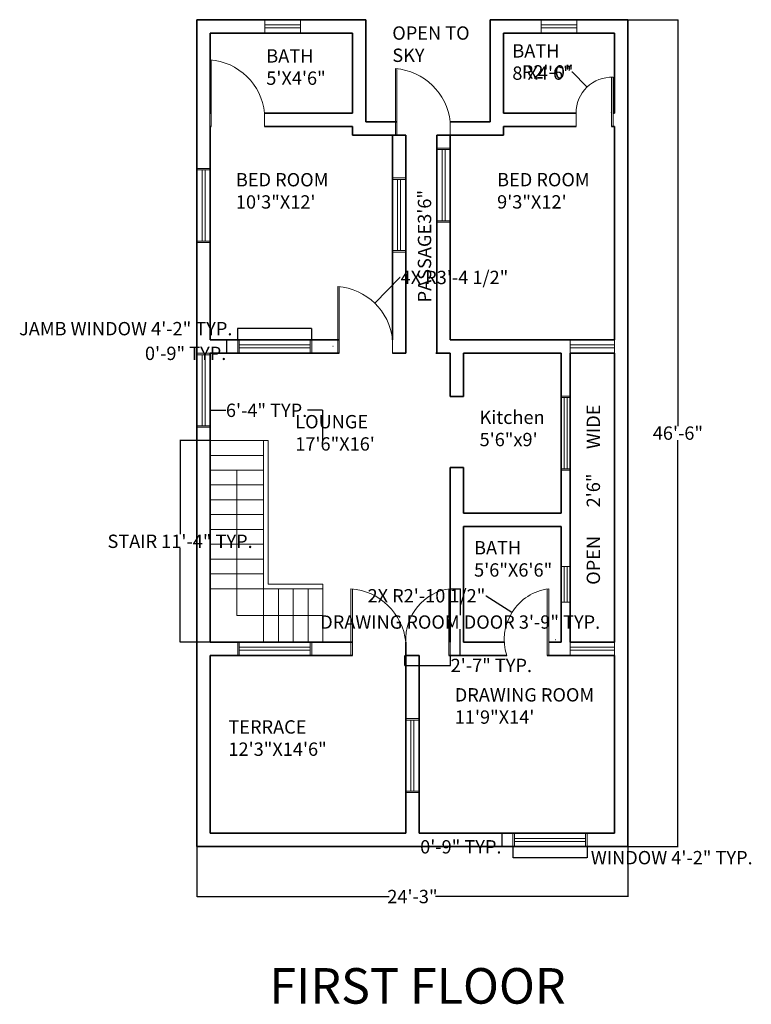
# Model space of a CAD drawing. Units: inches. Extents: x -56 to 1055, y -798 to 815.
# Tile 2 of 2: x 561 to 1055, y -756 to -91. Entities that reach past the tile are written whole.
import ezdxf

# ---------------------------------------------------------------- set-up
doc = ezdxf.new("R2010")
doc.units = ezdxf.units.IN
doc.header["$MEASUREMENT"] = 0
for name, color, linetype, lineweight in [('A-ANNO-DIMS', 2, 'Continuous', 18), ('A-ANNO-TEXT', 7, 'Continuous', 18), ('A-AREA-IDEN', 7, 'Continuous', 18), ('A-DOOR', 3, 'Continuous', 18), ('A-FLOR-STRS', 7, 'Continuous', 18), ('A-GLAZ', 4, 'Continuous', 18), ('A-WALL', 7, 'Continuous', 35)]:
    doc.layers.add(name, color=color, linetype=linetype, lineweight=lineweight)
doc.styles.get("Standard").update_dxf_attribs({"font": 'arial.ttf'})
doc.dimstyles.get("Standard").update_dxf_attribs({"dimtxt": 9, "dimasz": 0.18, "dimexe": 0.18, "dimexo": 0.0625, "dimgap": 0.09, "dimtad": 0, "dimtih": 1, "dimtoh": 1, "dimdec": 0, "dimzin": 0, "dimdsep": 46, "dimlunit": 3, "dimtxsty": 'Standard', "dimcen": 0.09, "dimadec": 0, "dimazin": 0, "dimtfac": 1, "dimtdec": 0, "dimtofl": 0, "dimtmove": 0, "dimatfit": 3, "dimfxl": 1, "dimtolj": 1, "dimtzin": 0, "dimarcsym": 0})

# ---------------------------------------------------------------- blocks, each defined once
blk = doc.blocks.new('door')
for p, q in [((432.11, -633.03), (432.11, -588.03)), ((433.11, -633.03), (433.11, -588.03)), ((469.11, -624.03), (469.11, -633.03))]:
    blk.add_line(p, q)
blk.add_arc((428.9, -628.35), 40.45, 6.12759, 85.44206)
blk = doc.blocks.new('WIN-50-FRAMED')
for p, q in [((0, 50), (9, 50)), ((0, 0), (0, 50)), ((0, 49), (9, 49)), ((3.5, 1), (3.5, 49)), ((5.5, 1), (5.5, 49)), ((9, 0), (9, 50)), ((0, 1), (9, 1)), ((0, 0), (9, 0))]:
    blk.add_line(p, q)
blk = doc.blocks.new('WIN-50-JAMB')
for p, q in [((0, 0), (0, 9)), ((1, 0), (1, 9)), ((49, 0), (49, 9)), ((50, 0), (50, 9)), ((1, 5.5), (49, 5.5)), ((1, 3.5), (49, 3.5))]:
    blk.add_line(p, q)
blk = doc.blocks.new('WIN-50-NARROW-WALL')
for p, q in [((0, 50), (6, 50)), ((0, 49), (6, 49)), ((2, 49), (2, 1)), ((4, 49), (4, 1)), ((0, 1), (6, 1)), ((0, 0), (6, 0))]:
    blk.add_line(p, q)
blk = doc.blocks.new('WIN-24-NARROW-WALL')
for p, q in [((0, 24), (6, 24)), ((2, 24), (2, 0)), ((4, 24), (4, 0)), ((0, 0), (6, 0))]:
    blk.add_line(p, q)
blk = doc.blocks.new('WIN-24-VENT')
for p, q in [((0, 0), (0, 9)), ((24, 0), (24, 9)), ((0, 5.5), (24, 5.5)), ((0, 3.5), (24, 3.5))]:
    blk.add_line(p, q)
blk = doc.blocks.new('DOOR-BATH-FRONT')
for p, q in [((29.04, 0), (29.04, 45)), ((30.04, 0), (30.04, 45)), ((0.04, 9), (0.04, 12.42))]:
    blk.add_line(p, q)
blk.add_arc((34.59, 10.71), 34.59, 97.55718, 198.03398)
blk = doc.blocks.new('DOOR-BATH-REAR')
for p, q in [((24, 0), (24, 33.14)), ((25, 0), (25, 33.14)), ((0, 0), (0, 9.51))]:
    blk.add_line(p, q)
blk.add_arc((23.91, 9.26), 23.91, 87.38829, 180.61249)
blk = doc.blocks.new('DOOR-DRAWING-ROOM')
for p, q in [((29.04, 0), (29.04, 45)), ((30.04, 0), (30.04, 45))]:
    blk.add_line(p, q)
blk.add_arc((34.59, 10.71), 34.59, 97.55718, 182.83167)
blk = doc.blocks.new('STAIR-RETURN')
for p, q in [((36, 136), (0, 136)), ((36, 136), (36, 36)), ((36, 136), (39, 136)), ((39, 136), (39, 39)), ((36, 126), (0, 126)), ((36, 116), (0, 116)), ((18, 116), (18, 18)), ((36, 106), (0, 106)), ((36, 96), (0, 96)), ((36, 86), (0, 86)), ((36, 76), (0, 76)), ((36, 66), (0, 66)), ((36, 56), (0, 56)), ((36, 46), (0, 46)), ((36, 36), (0, 36)), ((76, 36), (36, 36)), ((36, 36), (36, 0)), ((76, 39), (39, 39)), ((46, 36), (46, 0)), ((56, 36), (56, 0)), ((66, 36), (66, 0)), ((76, 36), (76, 39)), ((76, 36), (76, 0)), ((18, 18), (76, 18))]:
    blk.add_line(p, q)
blk = doc.blocks.new('WIN-30-OPENING')
for p, q in [((0, 0), (0, 9)), ((30, 9), (30, 0)), ((0, 5.5), (30, 5.5)), ((0, 3.5), (30, 3.5))]:
    blk.add_line(p, q)
blk = doc.blocks.new('WIN-30-SILL')
for p, q in [((0, 0), (0, 9)), ((30, 9), (30, 0)), ((0, 5.5), (30, 5.5)), ((0, 3.5), (30, 3.5)), ((0, 0), (30, 0))]:
    blk.add_line(p, q)
blk = doc.blocks.new('*D15')
at = {"layer": 'A-ANNO-DIMS', "color": 0, "lineweight": -2, "transparency": 16777216}
for p, q in [((893.64, -649.22), (893.64, -656.84)), ((943.64, -649.22), (943.64, -656.84)), ((893.82, -656.66), (943.46, -656.66)), ((943.64, -656.66), (943.82, -656.66))]:
    blk.add_line(p, q, dxfattribs=at)
at = {"layer": 'A-ANNO-DIMS', "color": 0, "transparency": 16777216}
for points in [[(893.82, -656.63), (893.82, -656.69), (893.64, -656.66)], [(943.46, -656.63), (943.46, -656.69), (943.64, -656.66)]]:
    blk.add_solid(points, dxfattribs=at)
at = {"layer": 'Defpoints', "color": 0, "transparency": 16777216}
for p in [(893.64, -649.16), (943.64, -649.16), (943.64, -656.66)]:
    blk.add_point(p, dxfattribs=at)
at = {"layer": 'A-ANNO-DIMS', "color": 0, "transparency": 16777216, "insert": (1000.85, -656.66), "char_height": 9, "attachment_point": 5}
blk.add_mtext('\\A1;WINDOW 4\'-2" TYP.', dxfattribs=at)
blk = doc.blocks.new('*D16')
at = {"layer": 'A-ANNO-DIMS', "color": 0, "lineweight": -2, "transparency": 16777216}
for p, q in [((893.58, -640.16), (885.96, -640.16)), ((886.14, -640.34), (886.14, -648.98)), ((893.58, -649.16), (885.96, -649.16)), ((886.14, -649.34), (885.96, -649.34)), ((886.14, -649.16), (886.14, -649.34))]:
    blk.add_line(p, q, dxfattribs=at)
at = {"layer": 'A-ANNO-DIMS', "color": 0, "transparency": 16777216}
for points in [[(886.11, -640.34), (886.17, -640.34), (886.14, -640.16)], [(886.11, -648.98), (886.17, -648.98), (886.14, -649.16)]]:
    blk.add_solid(points, dxfattribs=at)
at = {"layer": 'Defpoints', "color": 0, "transparency": 16777216}
for p in [(893.64, -640.16), (886.14, -649.16), (893.64, -649.16)]:
    blk.add_point(p, dxfattribs=at)
at = {"layer": 'A-ANNO-DIMS', "color": 0, "transparency": 16777216, "insert": (858.44, -649.34), "char_height": 9, "attachment_point": 5}
blk.add_mtext('\\A1;0\'-9" TYP.', dxfattribs=at)
blk = doc.blocks.new('*D19')
at = {"layer": 'A-ANNO-DIMS', "color": 0, "lineweight": -2, "transparency": 16777216}
for p, q in [((707.81, -299.66), (707.63, -299.66)), ((707.81, -307.1), (707.81, -299.48)), ((757.63, -299.66), (707.99, -299.66)), ((757.81, -307.1), (757.81, -299.48))]:
    blk.add_line(p, q, dxfattribs=at)
at = {"layer": 'A-ANNO-DIMS', "color": 0, "transparency": 16777216}
for points in [[(707.99, -299.63), (707.99, -299.69), (707.81, -299.66)], [(757.63, -299.63), (757.63, -299.69), (757.81, -299.66)]]:
    blk.add_solid(points, dxfattribs=at)
at = {"layer": 'Defpoints', "color": 0, "transparency": 16777216}
for p in [(707.81, -299.66), (707.81, -307.16), (757.81, -307.16)]:
    blk.add_point(p, dxfattribs=at)
at = {"layer": 'A-ANNO-DIMS', "color": 0, "transparency": 16777216, "insert": (632.18, -299.66), "char_height": 9, "attachment_point": 5}
blk.add_mtext('\\A1;JAMB WINDOW 4\'-2" TYP.', dxfattribs=at)
blk = doc.blocks.new('*D20')
at = {"layer": 'A-ANNO-DIMS', "color": 0, "lineweight": -2, "transparency": 16777216}
for p, q in [((707.75, -307.16), (700.13, -307.16)), ((700.31, -307.34), (700.31, -315.98)), ((707.75, -316.16), (700.13, -316.16)), ((700.31, -316.34), (700.13, -316.34)), ((700.31, -316.16), (700.31, -316.34))]:
    blk.add_line(p, q, dxfattribs=at)
at = {"layer": 'A-ANNO-DIMS', "color": 0, "transparency": 16777216}
for points in [[(700.28, -307.34), (700.34, -307.34), (700.31, -307.16)], [(700.28, -315.98), (700.34, -315.98), (700.31, -316.16)]]:
    blk.add_solid(points, dxfattribs=at)
at = {"layer": 'Defpoints', "color": 0, "transparency": 16777216}
for p in [(707.81, -307.16), (700.31, -316.16), (707.81, -316.16)]:
    blk.add_point(p, dxfattribs=at)
at = {"layer": 'A-ANNO-DIMS', "color": 0, "transparency": 16777216, "insert": (672.61, -316.34), "char_height": 9, "attachment_point": 5}
blk.add_mtext('\\A1;0\'-9" TYP.', dxfattribs=at)
blk = doc.blocks.new('*D31')
at = {"layer": 'A-ANNO-DIMS', "color": 0, "lineweight": -2, "transparency": 16777216}
for p, q in [((851.33, -475.16), (858.2, -475.16)), ((858.02, -475.34), (858.02, -492.91)), ((858.02, -519.98), (858.02, -502.41)), ((851.33, -520.16), (858.2, -520.16))]:
    blk.add_line(p, q, dxfattribs=at)
at = {"layer": 'A-ANNO-DIMS', "color": 0, "transparency": 16777216}
for points in [[(857.99, -475.34), (858.05, -475.34), (858.02, -475.16)], [(857.99, -519.98), (858.05, -519.98), (858.02, -520.16)]]:
    blk.add_solid(points, dxfattribs=at)
at = {"layer": 'Defpoints', "color": 0, "transparency": 16777216}
for p in [(851.27, -475.16), (858.02, -475.16), (851.27, -520.16)]:
    blk.add_point(p, dxfattribs=at)
at = {"layer": 'A-ANNO-DIMS', "color": 0, "transparency": 16777216, "insert": (858.02, -497.66), "char_height": 9, "attachment_point": 5}
blk.add_mtext('\\A1;DRAWING ROOM DOOR 3\'-9" TYP.', dxfattribs=at)
blk = doc.blocks.new('*D32')
at = {"layer": 'A-ANNO-DIMS', "color": 0, "lineweight": -2, "transparency": 16777216}
for p, q in [((820.38, -520.22), (820.38, -527.09)), ((851.27, -520.22), (851.27, -527.09)), ((820.56, -526.91), (851.09, -526.91)), ((851.27, -526.91), (851.45, -526.91))]:
    blk.add_line(p, q, dxfattribs=at)
at = {"layer": 'A-ANNO-DIMS', "color": 0, "transparency": 16777216}
for points in [[(820.56, -526.88), (820.56, -526.94), (820.38, -526.91)], [(851.09, -526.88), (851.09, -526.94), (851.27, -526.91)]]:
    blk.add_solid(points, dxfattribs=at)
at = {"layer": 'Defpoints', "color": 0, "transparency": 16777216}
for p in [(820.38, -520.16), (851.27, -520.16), (851.27, -526.91)]:
    blk.add_point(p, dxfattribs=at)
at = {"layer": 'A-ANNO-DIMS', "color": 0, "transparency": 16777216, "insert": (879.04, -526.91), "char_height": 9, "attachment_point": 5}
blk.add_mtext('\\A1;2\'-7" TYP.', dxfattribs=at)
blk = doc.blocks.new('*D33')
at = {"layer": 'A-ANNO-DIMS', "color": 0, "lineweight": -2, "transparency": 16777216}
for p, q in [((689.2, -375.16), (668.69, -375.16)), ((668.87, -375.34), (668.87, -438.42)), ((668.87, -510.98), (668.87, -447.9)), ((689.2, -511.16), (668.69, -511.16))]:
    blk.add_line(p, q, dxfattribs=at)
at = {"layer": 'A-ANNO-DIMS', "color": 0, "transparency": 16777216}
for points in [[(668.84, -375.34), (668.9, -375.34), (668.87, -375.16)], [(668.84, -510.98), (668.9, -510.98), (668.87, -511.16)]]:
    blk.add_solid(points, dxfattribs=at)
at = {"layer": 'Defpoints', "color": 0, "transparency": 16777216}
for p in [(668.87, -375.16), (689.27, -375.16), (689.27, -511.16)]:
    blk.add_point(p, dxfattribs=at)
at = {"layer": 'A-ANNO-DIMS', "color": 0, "transparency": 16777216, "insert": (668.87, -443.16), "char_height": 9, "attachment_point": 5}
blk.add_mtext('\\A1;STAIR 11\'-4" TYP.', dxfattribs=at)
blk = doc.blocks.new('*D34')
at = {"layer": 'A-ANNO-DIMS', "color": 0, "lineweight": -2, "transparency": 16777216}
for p, q in [((689.27, -375.1), (689.27, -354.58)), ((689.45, -354.76), (699.72, -354.76)), ((765.09, -354.76), (754.81, -354.76)), ((765.27, -375.1), (765.27, -354.58))]:
    blk.add_line(p, q, dxfattribs=at)
at = {"layer": 'A-ANNO-DIMS', "color": 0, "transparency": 16777216}
for points in [[(689.45, -354.73), (689.45, -354.79), (689.27, -354.76)], [(765.09, -354.73), (765.09, -354.79), (765.27, -354.76)]]:
    blk.add_solid(points, dxfattribs=at)
at = {"layer": 'Defpoints', "color": 0, "transparency": 16777216}
for p in [(765.27, -354.76), (689.27, -375.16), (765.27, -375.16)]:
    blk.add_point(p, dxfattribs=at)
at = {"layer": 'A-ANNO-DIMS', "color": 0, "transparency": 16777216, "insert": (727.27, -354.76), "char_height": 9, "attachment_point": 5}
blk.add_mtext('\\A1;6\'-4" TYP.', dxfattribs=at)
blk = doc.blocks.new('*D41')
at = {"layer": 'A-ANNO-DIMS', "color": 0, "lineweight": -2, "transparency": 16777216}
for p, q in [((680.27, -649.22), (680.27, -683.09)), ((971.27, -649.22), (971.27, -683.09)), ((680.45, -682.91), (810.14, -682.91)), ((971.09, -682.91), (841.39, -682.91))]:
    blk.add_line(p, q, dxfattribs=at)
at = {"layer": 'A-ANNO-DIMS', "color": 0, "transparency": 16777216}
for points in [[(680.45, -682.88), (680.45, -682.94), (680.27, -682.91)], [(971.09, -682.88), (971.09, -682.94), (971.27, -682.91)]]:
    blk.add_solid(points, dxfattribs=at)
at = {"layer": 'Defpoints', "color": 0, "transparency": 16777216}
for p in [(680.27, -649.16), (971.27, -649.16), (971.27, -682.91)]:
    blk.add_point(p, dxfattribs=at)
at = {"layer": 'A-ANNO-DIMS', "color": 0, "transparency": 16777216, "insert": (825.77, -682.91), "char_height": 9, "attachment_point": 5}
blk.add_mtext('\\A1;24\'-3"', dxfattribs=at)
blk = doc.blocks.new('*D42')
at = {"layer": 'A-ANNO-DIMS', "color": 0, "lineweight": -2, "transparency": 16777216}
for p, q in [((971.33, -91.16), (1005.2, -91.16)), ((1005.02, -91.34), (1005.02, -365.47)), ((1005.02, -648.98), (1005.02, -374.84)), ((971.33, -649.16), (1005.2, -649.16))]:
    blk.add_line(p, q, dxfattribs=at)
at = {"layer": 'A-ANNO-DIMS', "color": 0, "transparency": 16777216}
for points in [[(1004.99, -91.34), (1005.05, -91.34), (1005.02, -91.16)], [(1004.99, -648.98), (1005.05, -648.98), (1005.02, -649.16)]]:
    blk.add_solid(points, dxfattribs=at)
at = {"layer": 'Defpoints', "color": 0, "transparency": 16777216}
for p in [(971.27, -91.16), (971.27, -649.16), (1005.02, -649.16)]:
    blk.add_point(p, dxfattribs=at)
at = {"layer": 'A-ANNO-DIMS', "color": 0, "transparency": 16777216, "insert": (1005.02, -370.16), "char_height": 9, "attachment_point": 5}
blk.add_mtext('\\A1;46\'-6"', dxfattribs=at)
blk = doc.blocks.new('*D47')
at = {"layer": 'A-ANNO-DIMS', "color": 0, "lineweight": -2, "transparency": 16777216}
for p, q in [((817.27, -265.1), (800.47, -282.36)), ((817.45, -265.1), (817.27, -265.1)), ((772.05, -311.48), (772.23, -311.48)), ((772.14, -311.57), (772.14, -311.39))]:
    blk.add_line(p, q, dxfattribs=at)
at = {"layer": 'A-ANNO-DIMS', "color": 0, "transparency": 16777216}
blk.add_solid([(800.45, -282.34), (800.49, -282.38), (800.34, -282.49)], dxfattribs=at)
at = {"layer": 'Defpoints', "color": 0, "transparency": 16777216}
for p in [(800.34, -282.49), (772.14, -311.48)]:
    blk.add_point(p, dxfattribs=at)
at = {"layer": 'A-ANNO-DIMS', "color": 0, "transparency": 16777216, "insert": (854.14, -265.1), "char_height": 9, "attachment_point": 5}
blk.add_mtext('\\A1;4X R3\'-4 1/2"', dxfattribs=at)
blk = doc.blocks.new('*D48')
at = {"layer": 'A-ANNO-DIMS', "color": 0, "lineweight": -2, "transparency": 16777216}
for p, q in [((875.32, -479.95), (875.5, -479.95)), ((875.5, -479.95), (892.91, -490.92)), ((922.24, -509.45), (922.42, -509.45)), ((922.33, -509.54), (922.33, -509.36))]:
    blk.add_line(p, q, dxfattribs=at)
at = {"layer": 'A-ANNO-DIMS', "color": 0, "transparency": 16777216}
blk.add_solid([(892.92, -490.89), (892.89, -490.94), (893.06, -491.01)], dxfattribs=at)
at = {"layer": 'Defpoints', "color": 0, "transparency": 16777216}
for p in [(893.06, -491.01), (922.33, -509.45)]:
    blk.add_point(p, dxfattribs=at)
at = {"layer": 'A-ANNO-DIMS', "color": 0, "transparency": 16777216, "insert": (835.23, -479.95), "char_height": 9, "attachment_point": 5}
blk.add_mtext('\\A1;2X R2\'-10 1/2"', dxfattribs=at)
blk = doc.blocks.new('*D49')
at = {"layer": 'A-ANNO-DIMS', "color": 0, "lineweight": -2, "transparency": 16777216}
for p, q in [((933.43, -126.38), (933.61, -126.38)), ((933.61, -126.38), (943.45, -136.57)), ((960.1, -153.9), (960.28, -153.9)), ((960.19, -153.99), (960.19, -153.81))]:
    blk.add_line(p, q, dxfattribs=at)
at = {"layer": 'A-ANNO-DIMS', "color": 0, "transparency": 16777216}
blk.add_solid([(943.47, -136.55), (943.43, -136.59), (943.58, -136.7)], dxfattribs=at)
at = {"layer": 'Defpoints', "color": 0, "transparency": 16777216}
for p in [(943.58, -136.7), (960.19, -153.9)]:
    blk.add_point(p, dxfattribs=at)
at = {"layer": 'A-ANNO-DIMS', "color": 0, "transparency": 16777216, "insert": (917.07, -126.38), "char_height": 9, "attachment_point": 5}
blk.add_mtext('\\A1;R2\'-0"', dxfattribs=at)

msp = doc.modelspace()

# ---------------------------------------------------------------- linework, layer by layer
at = {"layer": 'A-WALL'}
for p, q in [((680.27, -91.16), (794.27, -91.16)), ((680.27, -91.16), (680.27, -649.16)), ((794.27, -91.16), (794.27, -160.16)), ((878.27, -91.16), (971.27, -91.16)), ((878.27, -91.16), (878.27, -160.16)), ((971.27, -91.16), (971.27, -649.16)), ((689.27, -100.16), (785.27, -100.16)), ((689.27, -100.16), (689.27, -154.16)), ((785.27, -100.16), (785.27, -154.16)), ((887.27, -100.16), (962.27, -100.16)), ((887.27, -100.16), (887.27, -154.16)), ((962.27, -100.16), (962.27, -154.16)), ((689.27, -154.16), (689.95, -154.16)), ((725.95, -154.16), (785.27, -154.16)), ((887.27, -154.16), (936.28, -154.16)), ((962.27, -154.16), (961.28, -154.02)), ((961.28, -154.16), (962.27, -154.16)), ((689.27, -163.16), (689.95, -163.16)), ((689.27, -163.16), (689.27, -307.16)), ((725.95, -163.16), (785.27, -163.16)), ((785.27, -163.16), (785.27, -169.16)), ((794.27, -160.16), (815.27, -160.16)), ((851.27, -160.16), (878.27, -160.16)), ((887.27, -163.16), (936.28, -163.16)), ((887.27, -169.16), (887.27, -163.16)), ((960.28, -163.16), (962.27, -163.16)), ((962.27, -163.16), (962.27, -307.16)), ((785.27, -169.16), (821.27, -169.16)), ((812.27, -169.16), (812.27, -307.16)), ((821.27, -169.16), (821.27, -316.16)), ((842.27, -169.16), (887.27, -169.16)), ((842.27, -169.16), (842.27, -316.16)), ((851.27, -169.16), (863.27, -169.16)), ((851.27, -169.16), (851.27, -307.16)), ((689.27, -307.16), (776.35, -307.16)), ((851.27, -307.16), (962.27, -307.16)), ((689.27, -316.16), (776.35, -316.16)), ((689.27, -316.16), (689.27, -511.16)), ((812.35, -316.16), (821.27, -316.16)), ((851.27, -316.16), (841.6, -316.16)), ((851.27, -316.16), (851.27, -345.36)), ((860.27, -316.16), (860.27, -345.36)), ((863.27, -316.16), (860.27, -316.16)), ((863.27, -316.16), (926.27, -316.16)), ((926.27, -316.16), (926.27, -424.16)), ((932.27, -316.16), (962.27, -316.16)), ((932.27, -316.16), (932.27, -433.16)), ((962.27, -316.16), (962.27, -511.16)), ((851.27, -345.36), (860.27, -345.36)), ((851.27, -393.36), (860.27, -393.36)), ((851.27, -393.36), (851.27, -511.16)), ((860.27, -393.36), (860.27, -424.16)), ((860.27, -424.16), (926.27, -424.16)), ((860.27, -433.16), (926.27, -433.16)), ((860.27, -433.16), (860.27, -511.16)), ((926.27, -433.16), (926.27, -511.16)), ((932.27, -433.16), (932.27, -511.16)), ((785.27, -511.16), (689.27, -511.16)), ((821.27, -511.16), (821.27, -640.16)), ((860.27, -511.16), (887.78, -511.16)), ((917.78, -511.16), (926.27, -511.16)), ((932.27, -511.16), (962.27, -511.16)), ((785.27, -520.16), (689.27, -520.16)), ((689.27, -520.16), (689.27, -640.16)), ((830.27, -520.16), (821.27, -520.16)), ((830.27, -520.16), (830.27, -640.16)), ((851.27, -520.16), (850.27, -520.16)), ((851.27, -520.16), (889.44, -520.16)), ((916.78, -520.16), (962.27, -520.16)), ((962.27, -520.16), (962.27, -640.16)), ((821.27, -640.16), (821.27, -604.16)), ((830.34, -640.16), (830.34, -604.16)), ((821.27, -640.16), (689.27, -640.16)), ((962.27, -640.16), (830.27, -640.16)), ((831.34, -649.16), (680.27, -649.16)), ((971.27, -649.16), (830.34, -649.16))]:
    msp.add_line(p, q, dxfattribs=at)

# ---------------------------------------------------------------- block references
at = {"layer": 'A-DOOR'}
for name, p in [('door', (256.84, 469.87)), ('door', (382.15, 463.87)), ('DOOR-BATH-REAR', (936.28, -163.16)), ('door', (343.24, 316.87)), ('door', (352.15, 112.87)), ('DOOR-DRAWING-ROOM', (821.22, -520.16)), ('DOOR-BATH-FRONT', (887.74, -520.16))]:
    msp.add_blockref(name, p, dxfattribs=at)
at = {"layer": 'A-FLOR-STRS'}
msp.add_blockref('STAIR-RETURN', (689.27, -511.16), dxfattribs=at)
at = {"layer": 'A-GLAZ'}
for name, p in [('WIN-24-VENT', (726.14, -100.16)), ('WIN-24-VENT', (912.77, -100.16)), ('WIN-50-FRAMED', (842.27, -227.84)), ('WIN-50-FRAMED', (680.27, -241.57)), ('WIN-50-FRAMED', (812.27, -247.99)), ('WIN-50-FRAMED', (680.27, -366.23)), ('WIN-50-NARROW-WALL', (926.27, -395.16)), ('WIN-24-NARROW-WALL', (926.27, -484.16)), ('WIN-30-SILL', (932.27, -520.16))]:
    msp.add_blockref(name, p, dxfattribs=at)
for name, p, rotation in [('WIN-50-JAMB', (757.81, -307.16), 180), ('WIN-30-OPENING', (962.27, -307.16), 180), ('WIN-50-JAMB', (757.77, -511.16), 180), ('WIN-50-JAMB', (821.27, -562.8), 270.0000000000003), ('WIN-50-FRAMED', (893.64, -640.16), 269.9999999999994)]:
    msp.add_blockref(name, p, dxfattribs=dict(at, rotation=rotation))

# ---------------------------------------------------------------- texts
at = {"layer": 'A-ANNO-TEXT', "insert": (943.43, -472.52), "char_height": 9, "attachment_point": 1, "rotation": 90}
msp.add_mtext_dynamic_manual_height_columns('OPEN       2\'6"      WIDE', width=153.2574, gutter_width=1, heights=[0], dxfattribs=at)
at = {"layer": 'A-ANNO-TEXT', "insert": (729.11, -731.2), "char_height": 24, "attachment_point": 1}
msp.add_mtext_dynamic_manual_height_columns('FIRST FLOOR', width=240.7989, gutter_width=1, heights=[0], dxfattribs=at)
at = {"layer": 'A-AREA-IDEN', "char_height": 9, "attachment_point": 1}
for s, width, insert in [('OPEN TO SKY', 55.271, (812.17, -95.67)), ('BATH\\P5\'X4\'6"', 73.9291, (727.07, -111.11)), ('BATH\\P8\'X4\'6"', 57.336, (893.21, -107.72)), ('BED ROOM\\P10\'3"X12\'', 86.6235, (706.56, -194.66)), ('BED ROOM\\P9\'3"X12\'', 63.0941, (882.94, -194.61)), ('LOUNGE\\P17\'6"X16\'', 92.9805, (746.64, -357.95)), ('Kitchen\\P5\'6"x9\'', 50.4169, (871.1, -354.99)), ('BATH\\P5\'6"X6\'6"', 45.2259, (867.39, -443.01)), ('DRAWING ROOM\\P11\'9"X14\'', 98.021, (854.34, -542.28)), ('TERRACE\\P12\'3"X14\'6"', 98.5311, (701.5, -563.95))]:
    msp.add_mtext_dynamic_manual_height_columns(s, width=width, gutter_width=1, heights=[0], dxfattribs=dict(at, insert=insert))
at = {"layer": 'A-AREA-IDEN', "insert": (829.42, -281.95), "char_height": 9, "attachment_point": 1, "rotation": 90}
msp.add_mtext_dynamic_manual_height_columns('PASSAGE3\'6"', width=12.3522, gutter_width=1, heights=[0], dxfattribs=at)

# ---------------------------------------------------------------- dimensions: what is measured, and where the dimension line sits
at = {"layer": 'A-ANNO-DIMS'}
dim = msp.add_linear_dim(base=(1005.02, -649.16), p1=(971.27, -91.16), p2=(971.27, -649.16), angle=90, dimstyle='Standard', override={"dimdec": 1, "dimlfac": 1, "dimrnd": 0, "dimzin": 1, "dimdsep": 46, "dimlunit": 4, "dimfrac": 2}, dxfattribs=at)
dim.commit()
dim.dimension.update_dxf_attribs({"geometry": '*D42', "text_midpoint": (1005.02, -370.16)})
dim = msp.add_radius_dim(center=(960.19, -153.9), mpoint=(943.58, -136.7), dimstyle='Standard', override={"dimdec": 1, "dimlfac": 1, "dimrnd": 0, "dimzin": 1, "dimdsep": 46, "dimlunit": 4, "dimfrac": 2}, dxfattribs=at)
dim.commit()
dim.dimension.update_dxf_attribs({"geometry": '*D49', "text_midpoint": (917.07, -126.38), "dimtype": 164})
for center, mpoint, text, picture, middle in [((772.14, -311.48), (800.34, -282.49), '4X <>', '*D47', (854.14, -265.1)), ((922.33, -509.45), (893.06, -491.01), '2X <>', '*D48', (835.23, -479.95))]:
    dim = msp.add_radius_dim(center=center, mpoint=mpoint, text=text, dimstyle='Standard', override={"dimdec": 1, "dimlfac": 1, "dimrnd": 0, "dimzin": 1, "dimdsep": 46, "dimlunit": 4, "dimfrac": 2}, dxfattribs=at)
    dim.commit()
    dim.dimension.update_dxf_attribs({"geometry": picture, "text_midpoint": middle, "dimtype": 164})
for base, p1, p2, angle, text, picture, middle in [((707.81, -299.66), (757.81, -307.16), (707.81, -307.16), 180, 'JAMB WINDOW <> TYP.', '*D19', (632.18, -299.66)), ((700.31, -316.16), (707.81, -307.16), (707.81, -316.16), 270, '<> TYP.', '*D20', (672.61, -316.34)), ((668.87, -375.16), (689.27, -511.16), (689.27, -375.16), 90, 'STAIR <> TYP.', '*D33', (668.87, -443.16)), ((858.02, -475.16), (851.27, -520.16), (851.27, -475.16), 90, 'DRAWING ROOM DOOR <> TYP.', '*D31', (858.02, -497.66)), ((886.14, -649.16), (893.64, -640.16), (893.64, -649.16), 270, '<> TYP.', '*D16', (858.44, -649.34))]:
    dim = msp.add_linear_dim(base=base, p1=p1, p2=p2, angle=angle, text=text, dimstyle='Standard', override={"dimdec": 1, "dimlfac": 1, "dimrnd": 0, "dimzin": 1, "dimdsep": 46, "dimlunit": 4, "dimfrac": 2}, dxfattribs=at)
    dim.commit()
    dim.dimension.update_dxf_attribs({"geometry": picture, "text_midpoint": middle})
for base, p1, p2, text, picture, middle in [((765.27, -354.76), (689.27, -375.16), (765.27, -375.16), '<> TYP.', '*D34', (727.27, -354.76)), ((851.27, -526.91), (820.38, -520.16), (851.27, -520.16), '<> TYP.', '*D32', (879.04, -526.91)), ((943.64, -656.66), (893.64, -649.16), (943.64, -649.16), 'WINDOW <> TYP.', '*D15', (1000.85, -656.66))]:
    dim = msp.add_linear_dim(base=base, p1=p1, p2=p2, text=text, dimstyle='Standard', override={"dimdec": 1, "dimlfac": 1, "dimrnd": 0, "dimzin": 1, "dimdsep": 46, "dimlunit": 4, "dimfrac": 2}, dxfattribs=at)
    dim.commit()
    dim.dimension.update_dxf_attribs({"geometry": picture, "text_midpoint": middle})
dim = msp.add_linear_dim(base=(971.27, -682.91), p1=(680.27, -649.16), p2=(971.27, -649.16), dimstyle='Standard', override={"dimdec": 1, "dimlfac": 1, "dimrnd": 0, "dimzin": 1, "dimdsep": 46, "dimlunit": 4, "dimfrac": 2}, dxfattribs=at)
dim.commit()
dim.dimension.update_dxf_attribs({"geometry": '*D41', "text_midpoint": (825.77, -682.91)})

doc.saveas('drawing.dxf')
